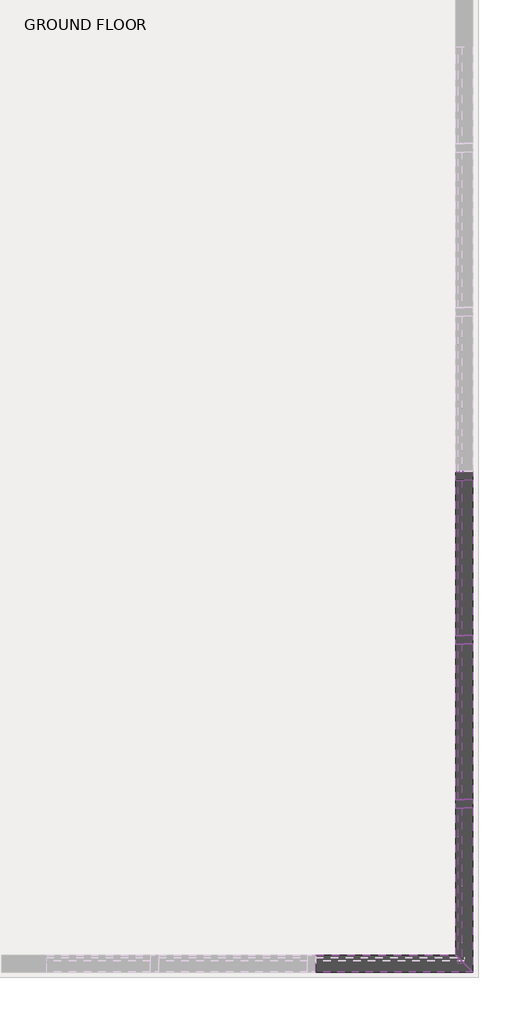
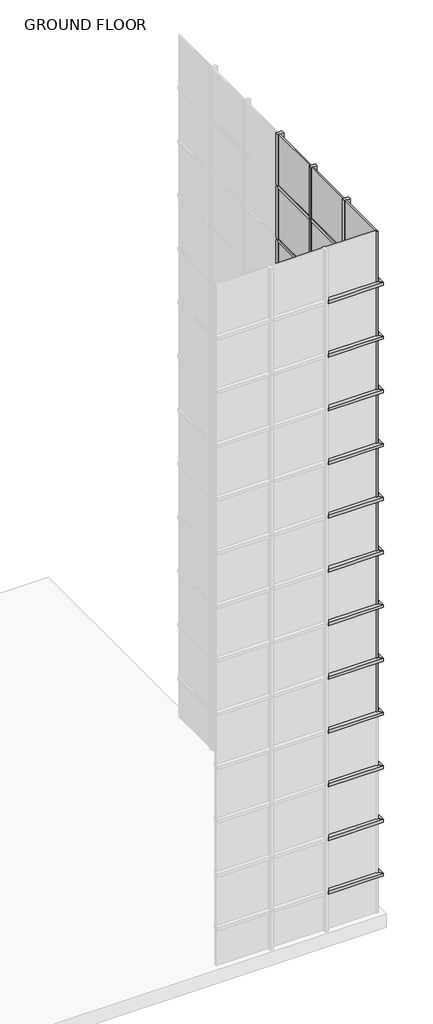
# One storey, part 6 of 16: 87 members, 43 plates.
"""IFC4 building model written with IfcOpenShell, lengths in millimetres."""

from ifc_helpers import new_model, si_unit, origin, place, context, project, spatial, transform, mapped, element, save
from components import member_a361ce75, member_80100a85, member_b860638c, member_31fee25f, member_49b1bc66, system_panel_glazed_49652e9e

model = new_model("IFC4")

# Units and contexts
model_context = context("Model", 3, world=origin())
ifc_project = project(units=[si_unit("LENGTHUNIT", "METRE", prefix="MILLI")], contexts=[model_context])

# Site, building, storey
site = spatial("IfcSite", under=ifc_project)
building = spatial("IfcBuilding", under=site)
storey = spatial("IfcBuildingStorey", under=building, Name="GROUND FLOOR", Elevation=0.0)

# Members
placement = place(None, origin())
member_shape = member_a361ce75(model_context)
element("IfcMember", 1, ObjectType="Rectangular Mullion : 2.5\" x 5\" rectangular", at=placement, inside=storey, context=model_context, shape_type="MappedRepresentation", body=[
    mapped(member_shape, transform((5962.6982466, -5739.2238032, 1168.8884615), x_axis=(0.0, 0.0, 1.0), y_axis=(0.0, -1.0, 0.0), z_axis=(1.0, 0.0, 0.0))),
])
element("IfcMember", 2, ObjectType="Rectangular Mullion : 2.5\" x 5\" rectangular", at=placement, inside=storey, context=model_context, shape_type="MappedRepresentation", body=[
    mapped(member_shape, transform((5962.6982466, -5739.2238032, 2369.5269231), x_axis=(0.0, 0.0, 1.0), y_axis=(0.0, -1.0, 0.0), z_axis=(1.0, 0.0, 0.0))),
])
element("IfcMember", 3, ObjectType="Rectangular Mullion : 2.5\" x 5\" rectangular", at=placement, inside=storey, context=model_context, shape_type="MappedRepresentation", body=[
    mapped(member_shape, transform((5962.6982466, -5739.2238032, 3570.1653846), x_axis=(0.0, 0.0, 1.0), y_axis=(0.0, -1.0, 0.0), z_axis=(1.0, 0.0, 0.0))),
])
element("IfcMember", 4, ObjectType="Rectangular Mullion : 2.5\" x 5\" rectangular", at=placement, inside=storey, context=model_context, shape_type="MappedRepresentation", body=[
    mapped(member_shape, transform((5962.6982466, -5739.2238032, 4770.8038462), x_axis=(0.0, 0.0, 1.0), y_axis=(0.0, -1.0, 0.0), z_axis=(1.0, 0.0, 0.0))),
])
element("IfcMember", 5, ObjectType="Rectangular Mullion : 2.5\" x 5\" rectangular", at=placement, inside=storey, context=model_context, shape_type="MappedRepresentation", body=[
    mapped(member_shape, transform((5962.6982466, -5739.2238032, 5971.4423077), x_axis=(0.0, 0.0, 1.0), y_axis=(0.0, -1.0, 0.0), z_axis=(1.0, 0.0, 0.0))),
])
element("IfcMember", 6, ObjectType="Rectangular Mullion : 2.5\" x 5\" rectangular", at=placement, inside=storey, context=model_context, shape_type="MappedRepresentation", body=[
    mapped(member_shape, transform((5962.6982466, -5739.2238032, 7172.0807692), x_axis=(0.0, 0.0, 1.0), y_axis=(0.0, -1.0, 0.0), z_axis=(1.0, 0.0, 0.0))),
])
element("IfcMember", 7, ObjectType="Rectangular Mullion : 2.5\" x 5\" rectangular", at=placement, inside=storey, context=model_context, shape_type="MappedRepresentation", body=[
    mapped(member_shape, transform((5962.6982466, -5739.2238032, 8372.7192308), x_axis=(0.0, 0.0, 1.0), y_axis=(0.0, -1.0, 0.0), z_axis=(1.0, 0.0, 0.0))),
])
element("IfcMember", 8, ObjectType="Rectangular Mullion : 2.5\" x 5\" rectangular", at=placement, inside=storey, context=model_context, shape_type="MappedRepresentation", body=[
    mapped(member_shape, transform((5962.6982466, -5739.2238032, 9573.3576923), x_axis=(0.0, 0.0, 1.0), y_axis=(0.0, -1.0, 0.0), z_axis=(1.0, 0.0, 0.0))),
])
element("IfcMember", 9, ObjectType="Rectangular Mullion : 2.5\" x 5\" rectangular", at=placement, inside=storey, context=model_context, shape_type="MappedRepresentation", body=[
    mapped(member_shape, transform((5962.6982466, -5739.2238032, 10773.9961538), x_axis=(0.0, 0.0, 1.0), y_axis=(0.0, -1.0, 0.0), z_axis=(1.0, 0.0, 0.0))),
])
element("IfcMember", 10, ObjectType="Rectangular Mullion : 2.5\" x 5\" rectangular", at=placement, inside=storey, context=model_context, shape_type="MappedRepresentation", body=[
    mapped(member_shape, transform((5962.6982466, -5739.2238032, 11974.6346154), x_axis=(0.0, 0.0, 1.0), y_axis=(0.0, -1.0, 0.0), z_axis=(1.0, 0.0, 0.0))),
])
element("IfcMember", 11, ObjectType="Rectangular Mullion : 2.5\" x 5\" rectangular", at=placement, inside=storey, context=model_context, shape_type="MappedRepresentation", body=[
    mapped(member_shape, transform((5962.6982466, -5739.2238032, 13175.2730769), x_axis=(0.0, 0.0, 1.0), y_axis=(0.0, -1.0, 0.0), z_axis=(1.0, 0.0, 0.0))),
])
element("IfcMember", 12, ObjectType="Rectangular Mullion : 2.5\" x 5\" rectangular", at=placement, inside=storey, context=model_context, shape_type="MappedRepresentation", body=[
    mapped(member_shape, transform((5962.6982466, -5739.2238032, 14375.9115385), x_axis=(0.0, 0.0, 1.0), y_axis=(0.0, -1.0, 0.0), z_axis=(1.0, 0.0, 0.0))),
])
member_2_shape = member_80100a85(model_context)
element("IfcMember", 13, ObjectType="Rectangular Mullion : 2.5\" x 5\" rectangular", at=placement, inside=storey, context=model_context, shape_type="MappedRepresentation", body=[
    mapped(member_2_shape, transform((5962.6982466, -4585.428803, 1168.8884615), x_axis=(0.0, 0.0, 1.0), y_axis=(1.0, 0.0, 0.0), z_axis=(0.0, 1.0, 0.0))),
])
element("IfcMember", 14, ObjectType="Rectangular Mullion : 2.5\" x 5\" rectangular", at=placement, inside=storey, context=model_context, shape_type="MappedRepresentation", body=[
    mapped(member_2_shape, transform((5962.6982466, -4585.428803, 2369.5269231), x_axis=(0.0, 0.0, 1.0), y_axis=(1.0, 0.0, 0.0), z_axis=(0.0, 1.0, 0.0))),
])
element("IfcMember", 15, ObjectType="Rectangular Mullion : 2.5\" x 5\" rectangular", at=placement, inside=storey, context=model_context, shape_type="MappedRepresentation", body=[
    mapped(member_2_shape, transform((5962.6982466, -4585.428803, 3570.1653846), x_axis=(0.0, 0.0, 1.0), y_axis=(1.0, 0.0, 0.0), z_axis=(0.0, 1.0, 0.0))),
])
element("IfcMember", 16, ObjectType="Rectangular Mullion : 2.5\" x 5\" rectangular", at=placement, inside=storey, context=model_context, shape_type="MappedRepresentation", body=[
    mapped(member_2_shape, transform((5962.6982466, -4585.428803, 4770.8038462), x_axis=(0.0, 0.0, 1.0), y_axis=(1.0, 0.0, 0.0), z_axis=(0.0, 1.0, 0.0))),
])
element("IfcMember", 17, ObjectType="Rectangular Mullion : 2.5\" x 5\" rectangular", at=placement, inside=storey, context=model_context, shape_type="MappedRepresentation", body=[
    mapped(member_2_shape, transform((5962.6982466, -4585.428803, 5971.4423077), x_axis=(0.0, 0.0, 1.0), y_axis=(1.0, 0.0, 0.0), z_axis=(0.0, 1.0, 0.0))),
])
element("IfcMember", 18, ObjectType="Rectangular Mullion : 2.5\" x 5\" rectangular", at=placement, inside=storey, context=model_context, shape_type="MappedRepresentation", body=[
    mapped(member_2_shape, transform((5962.6982466, -4585.428803, 7172.0807692), x_axis=(0.0, 0.0, 1.0), y_axis=(1.0, 0.0, 0.0), z_axis=(0.0, 1.0, 0.0))),
])
element("IfcMember", 19, ObjectType="Rectangular Mullion : 2.5\" x 5\" rectangular", at=placement, inside=storey, context=model_context, shape_type="MappedRepresentation", body=[
    mapped(member_2_shape, transform((5962.6982466, -4585.428803, 8372.7192308), x_axis=(0.0, 0.0, 1.0), y_axis=(1.0, 0.0, 0.0), z_axis=(0.0, 1.0, 0.0))),
])
element("IfcMember", 20, ObjectType="Rectangular Mullion : 2.5\" x 5\" rectangular", at=placement, inside=storey, context=model_context, shape_type="MappedRepresentation", body=[
    mapped(member_2_shape, transform((5962.6982466, -4585.428803, 9573.3576923), x_axis=(0.0, 0.0, 1.0), y_axis=(1.0, 0.0, 0.0), z_axis=(0.0, 1.0, 0.0))),
])
element("IfcMember", 21, ObjectType="Rectangular Mullion : 2.5\" x 5\" rectangular", at=placement, inside=storey, context=model_context, shape_type="MappedRepresentation", body=[
    mapped(member_2_shape, transform((5962.6982466, -4585.428803, 10773.9961538), x_axis=(0.0, 0.0, 1.0), y_axis=(1.0, 0.0, 0.0), z_axis=(0.0, 1.0, 0.0))),
])
element("IfcMember", 22, ObjectType="Rectangular Mullion : 2.5\" x 5\" rectangular", at=placement, inside=storey, context=model_context, shape_type="MappedRepresentation", body=[
    mapped(member_2_shape, transform((5962.6982466, -4585.428803, 11974.6346154), x_axis=(0.0, 0.0, 1.0), y_axis=(1.0, 0.0, 0.0), z_axis=(0.0, 1.0, 0.0))),
])
element("IfcMember", 23, ObjectType="Rectangular Mullion : 2.5\" x 5\" rectangular", at=placement, inside=storey, context=model_context, shape_type="MappedRepresentation", body=[
    mapped(member_2_shape, transform((5962.6982466, -4585.428803, 13175.2730769), x_axis=(0.0, 0.0, 1.0), y_axis=(1.0, 0.0, 0.0), z_axis=(0.0, 1.0, 0.0))),
])
element("IfcMember", 24, ObjectType="Rectangular Mullion : 2.5\" x 5\" rectangular", at=placement, inside=storey, context=model_context, shape_type="MappedRepresentation", body=[
    mapped(member_2_shape, transform((5962.6982466, -4585.428803, 14375.9115385), x_axis=(0.0, 0.0, 1.0), y_axis=(1.0, 0.0, 0.0), z_axis=(0.0, 1.0, 0.0))),
])
member_3_shape = member_b860638c(model_context)
element("IfcMember", 25, ObjectType="Rectangular Mullion : 2.5\" x 5\" rectangular", at=placement, inside=storey, context=model_context, shape_type="MappedRepresentation", body=[
    mapped(member_3_shape, transform((5962.6982466, -4553.678803, 0.0), x_axis=(0.0, 1.0, 0.0), y_axis=(1.0, 0.0, 0.0), z_axis=(0.0, 0.0, -1.0))),
])
element("IfcMember", 26, ObjectType="Rectangular Mullion : 2.5\" x 5\" rectangular", at=placement, inside=storey, context=model_context, shape_type="MappedRepresentation", body=[
    mapped(member_3_shape, transform((5962.6982466, -3336.383803, 0.0), x_axis=(0.0, 1.0, 0.0), y_axis=(1.0, 0.0, 0.0), z_axis=(0.0, 0.0, -1.0))),
])
element("IfcMember", 27, ObjectType="Rectangular Mullion : 2.5\" x 5\" rectangular", at=placement, inside=storey, context=model_context, shape_type="MappedRepresentation", body=[
    mapped(member_3_shape, transform((5962.6982466, -2119.0888031, 0.0), x_axis=(0.0, 1.0, 0.0), y_axis=(1.0, 0.0, 0.0), z_axis=(0.0, 0.0, -1.0))),
])
member_4_shape = member_31fee25f(model_context)
element("IfcMember", 28, ObjectType="Rectangular Mullion : 2.5\" x 5\" rectangular", at=placement, inside=storey, context=model_context, shape_type="MappedRepresentation", body=[
    mapped(member_4_shape, transform((5962.6982466, -4553.678803, 1168.8884615), x_axis=(0.0, 1.0, 0.0), y_axis=(1.0, 0.0, 0.0), z_axis=(0.0, 0.0, -1.0))),
])
element("IfcMember", 29, ObjectType="Rectangular Mullion : 2.5\" x 5\" rectangular", at=placement, inside=storey, context=model_context, shape_type="MappedRepresentation", body=[
    mapped(member_4_shape, transform((5962.6982466, -3336.383803, 1168.8884615), x_axis=(0.0, 1.0, 0.0), y_axis=(1.0, 0.0, 0.0), z_axis=(0.0, 0.0, -1.0))),
])
element("IfcMember", 30, ObjectType="Rectangular Mullion : 2.5\" x 5\" rectangular", at=placement, inside=storey, context=model_context, shape_type="MappedRepresentation", body=[
    mapped(member_4_shape, transform((5962.6982466, -2119.0888031, 1168.8884615), x_axis=(0.0, 1.0, 0.0), y_axis=(1.0, 0.0, 0.0), z_axis=(0.0, 0.0, -1.0))),
])
element("IfcMember", 31, ObjectType="Rectangular Mullion : 2.5\" x 5\" rectangular", at=placement, inside=storey, context=model_context, shape_type="MappedRepresentation", body=[
    mapped(member_4_shape, transform((5962.6982466, -4553.678803, 2369.5269231), x_axis=(0.0, 1.0, 0.0), y_axis=(1.0, 0.0, 0.0), z_axis=(0.0, 0.0, -1.0))),
])
element("IfcMember", 32, ObjectType="Rectangular Mullion : 2.5\" x 5\" rectangular", at=placement, inside=storey, context=model_context, shape_type="MappedRepresentation", body=[
    mapped(member_4_shape, transform((5962.6982466, -3336.383803, 2369.5269231), x_axis=(0.0, 1.0, 0.0), y_axis=(1.0, 0.0, 0.0), z_axis=(0.0, 0.0, -1.0))),
])
element("IfcMember", 33, ObjectType="Rectangular Mullion : 2.5\" x 5\" rectangular", at=placement, inside=storey, context=model_context, shape_type="MappedRepresentation", body=[
    mapped(member_4_shape, transform((5962.6982466, -2119.0888031, 2369.5269231), x_axis=(0.0, 1.0, 0.0), y_axis=(1.0, 0.0, 0.0), z_axis=(0.0, 0.0, -1.0))),
])
element("IfcMember", 34, ObjectType="Rectangular Mullion : 2.5\" x 5\" rectangular", at=placement, inside=storey, context=model_context, shape_type="MappedRepresentation", body=[
    mapped(member_4_shape, transform((5962.6982466, -4553.678803, 3570.1653846), x_axis=(0.0, 1.0, 0.0), y_axis=(1.0, 0.0, 0.0), z_axis=(0.0, 0.0, -1.0))),
])
element("IfcMember", 35, ObjectType="Rectangular Mullion : 2.5\" x 5\" rectangular", at=placement, inside=storey, context=model_context, shape_type="MappedRepresentation", body=[
    mapped(member_4_shape, transform((5962.6982466, -3336.383803, 3570.1653846), x_axis=(0.0, 1.0, 0.0), y_axis=(1.0, 0.0, 0.0), z_axis=(0.0, 0.0, -1.0))),
])
element("IfcMember", 36, ObjectType="Rectangular Mullion : 2.5\" x 5\" rectangular", at=placement, inside=storey, context=model_context, shape_type="MappedRepresentation", body=[
    mapped(member_4_shape, transform((5962.6982466, -2119.0888031, 3570.1653846), x_axis=(0.0, 1.0, 0.0), y_axis=(1.0, 0.0, 0.0), z_axis=(0.0, 0.0, -1.0))),
])
element("IfcMember", 37, ObjectType="Rectangular Mullion : 2.5\" x 5\" rectangular", at=placement, inside=storey, context=model_context, shape_type="MappedRepresentation", body=[
    mapped(member_4_shape, transform((5962.6982466, -4553.678803, 4770.8038462), x_axis=(0.0, 1.0, 0.0), y_axis=(1.0, 0.0, 0.0), z_axis=(0.0, 0.0, -1.0))),
])
element("IfcMember", 38, ObjectType="Rectangular Mullion : 2.5\" x 5\" rectangular", at=placement, inside=storey, context=model_context, shape_type="MappedRepresentation", body=[
    mapped(member_4_shape, transform((5962.6982466, -3336.383803, 4770.8038462), x_axis=(0.0, 1.0, 0.0), y_axis=(1.0, 0.0, 0.0), z_axis=(0.0, 0.0, -1.0))),
])
element("IfcMember", 39, ObjectType="Rectangular Mullion : 2.5\" x 5\" rectangular", at=placement, inside=storey, context=model_context, shape_type="MappedRepresentation", body=[
    mapped(member_4_shape, transform((5962.6982466, -2119.0888031, 4770.8038462), x_axis=(0.0, 1.0, 0.0), y_axis=(1.0, 0.0, 0.0), z_axis=(0.0, 0.0, -1.0))),
])
element("IfcMember", 40, ObjectType="Rectangular Mullion : 2.5\" x 5\" rectangular", at=placement, inside=storey, context=model_context, shape_type="MappedRepresentation", body=[
    mapped(member_4_shape, transform((5962.6982466, -4553.678803, 5971.4423077), x_axis=(0.0, 1.0, 0.0), y_axis=(1.0, 0.0, 0.0), z_axis=(0.0, 0.0, -1.0))),
])
element("IfcMember", 41, ObjectType="Rectangular Mullion : 2.5\" x 5\" rectangular", at=placement, inside=storey, context=model_context, shape_type="MappedRepresentation", body=[
    mapped(member_4_shape, transform((5962.6982466, -3336.383803, 5971.4423077), x_axis=(0.0, 1.0, 0.0), y_axis=(1.0, 0.0, 0.0), z_axis=(0.0, 0.0, -1.0))),
])
element("IfcMember", 42, ObjectType="Rectangular Mullion : 2.5\" x 5\" rectangular", at=placement, inside=storey, context=model_context, shape_type="MappedRepresentation", body=[
    mapped(member_4_shape, transform((5962.6982466, -2119.0888031, 5971.4423077), x_axis=(0.0, 1.0, 0.0), y_axis=(1.0, 0.0, 0.0), z_axis=(0.0, 0.0, -1.0))),
])
element("IfcMember", 43, ObjectType="Rectangular Mullion : 2.5\" x 5\" rectangular", at=placement, inside=storey, context=model_context, shape_type="MappedRepresentation", body=[
    mapped(member_4_shape, transform((5962.6982466, -4553.678803, 7172.0807692), x_axis=(0.0, 1.0, 0.0), y_axis=(1.0, 0.0, 0.0), z_axis=(0.0, 0.0, -1.0))),
])
element("IfcMember", 44, ObjectType="Rectangular Mullion : 2.5\" x 5\" rectangular", at=placement, inside=storey, context=model_context, shape_type="MappedRepresentation", body=[
    mapped(member_4_shape, transform((5962.6982466, -3336.383803, 7172.0807692), x_axis=(0.0, 1.0, 0.0), y_axis=(1.0, 0.0, 0.0), z_axis=(0.0, 0.0, -1.0))),
])
element("IfcMember", 45, ObjectType="Rectangular Mullion : 2.5\" x 5\" rectangular", at=placement, inside=storey, context=model_context, shape_type="MappedRepresentation", body=[
    mapped(member_4_shape, transform((5962.6982466, -2119.0888031, 7172.0807692), x_axis=(0.0, 1.0, 0.0), y_axis=(1.0, 0.0, 0.0), z_axis=(0.0, 0.0, -1.0))),
])
element("IfcMember", 46, ObjectType="Rectangular Mullion : 2.5\" x 5\" rectangular", at=placement, inside=storey, context=model_context, shape_type="MappedRepresentation", body=[
    mapped(member_4_shape, transform((5962.6982466, -4553.678803, 8372.7192308), x_axis=(0.0, 1.0, 0.0), y_axis=(1.0, 0.0, 0.0), z_axis=(0.0, 0.0, -1.0))),
])
element("IfcMember", 47, ObjectType="Rectangular Mullion : 2.5\" x 5\" rectangular", at=placement, inside=storey, context=model_context, shape_type="MappedRepresentation", body=[
    mapped(member_4_shape, transform((5962.6982466, -3336.383803, 8372.7192308), x_axis=(0.0, 1.0, 0.0), y_axis=(1.0, 0.0, 0.0), z_axis=(0.0, 0.0, -1.0))),
])
element("IfcMember", 48, ObjectType="Rectangular Mullion : 2.5\" x 5\" rectangular", at=placement, inside=storey, context=model_context, shape_type="MappedRepresentation", body=[
    mapped(member_4_shape, transform((5962.6982466, -2119.0888031, 8372.7192308), x_axis=(0.0, 1.0, 0.0), y_axis=(1.0, 0.0, 0.0), z_axis=(0.0, 0.0, -1.0))),
])
element("IfcMember", 49, ObjectType="Rectangular Mullion : 2.5\" x 5\" rectangular", at=placement, inside=storey, context=model_context, shape_type="MappedRepresentation", body=[
    mapped(member_4_shape, transform((5962.6982466, -4553.678803, 9573.3576923), x_axis=(0.0, 1.0, 0.0), y_axis=(1.0, 0.0, 0.0), z_axis=(0.0, 0.0, -1.0))),
])
element("IfcMember", 50, ObjectType="Rectangular Mullion : 2.5\" x 5\" rectangular", at=placement, inside=storey, context=model_context, shape_type="MappedRepresentation", body=[
    mapped(member_4_shape, transform((5962.6982466, -3336.383803, 9573.3576923), x_axis=(0.0, 1.0, 0.0), y_axis=(1.0, 0.0, 0.0), z_axis=(0.0, 0.0, -1.0))),
])
element("IfcMember", 51, ObjectType="Rectangular Mullion : 2.5\" x 5\" rectangular", at=placement, inside=storey, context=model_context, shape_type="MappedRepresentation", body=[
    mapped(member_4_shape, transform((5962.6982466, -2119.0888031, 9573.3576923), x_axis=(0.0, 1.0, 0.0), y_axis=(1.0, 0.0, 0.0), z_axis=(0.0, 0.0, -1.0))),
])
element("IfcMember", 52, ObjectType="Rectangular Mullion : 2.5\" x 5\" rectangular", at=placement, inside=storey, context=model_context, shape_type="MappedRepresentation", body=[
    mapped(member_4_shape, transform((5962.6982466, -4553.678803, 10773.9961538), x_axis=(0.0, 1.0, 0.0), y_axis=(1.0, 0.0, 0.0), z_axis=(0.0, 0.0, -1.0))),
])
element("IfcMember", 53, ObjectType="Rectangular Mullion : 2.5\" x 5\" rectangular", at=placement, inside=storey, context=model_context, shape_type="MappedRepresentation", body=[
    mapped(member_4_shape, transform((5962.6982466, -3336.383803, 10773.9961538), x_axis=(0.0, 1.0, 0.0), y_axis=(1.0, 0.0, 0.0), z_axis=(0.0, 0.0, -1.0))),
])
element("IfcMember", 54, ObjectType="Rectangular Mullion : 2.5\" x 5\" rectangular", at=placement, inside=storey, context=model_context, shape_type="MappedRepresentation", body=[
    mapped(member_4_shape, transform((5962.6982466, -2119.0888031, 10773.9961538), x_axis=(0.0, 1.0, 0.0), y_axis=(1.0, 0.0, 0.0), z_axis=(0.0, 0.0, -1.0))),
])
element("IfcMember", 55, ObjectType="Rectangular Mullion : 2.5\" x 5\" rectangular", at=placement, inside=storey, context=model_context, shape_type="MappedRepresentation", body=[
    mapped(member_4_shape, transform((5962.6982466, -4553.678803, 11974.6346154), x_axis=(0.0, 1.0, 0.0), y_axis=(1.0, 0.0, 0.0), z_axis=(0.0, 0.0, -1.0))),
])
element("IfcMember", 56, ObjectType="Rectangular Mullion : 2.5\" x 5\" rectangular", at=placement, inside=storey, context=model_context, shape_type="MappedRepresentation", body=[
    mapped(member_4_shape, transform((5962.6982466, -3336.383803, 11974.6346154), x_axis=(0.0, 1.0, 0.0), y_axis=(1.0, 0.0, 0.0), z_axis=(0.0, 0.0, -1.0))),
])
element("IfcMember", 57, ObjectType="Rectangular Mullion : 2.5\" x 5\" rectangular", at=placement, inside=storey, context=model_context, shape_type="MappedRepresentation", body=[
    mapped(member_4_shape, transform((5962.6982466, -2119.0888031, 11974.6346154), x_axis=(0.0, 1.0, 0.0), y_axis=(1.0, 0.0, 0.0), z_axis=(0.0, 0.0, -1.0))),
])
element("IfcMember", 58, ObjectType="Rectangular Mullion : 2.5\" x 5\" rectangular", at=placement, inside=storey, context=model_context, shape_type="MappedRepresentation", body=[
    mapped(member_4_shape, transform((5962.6982466, -4553.678803, 13175.2730769), x_axis=(0.0, 1.0, 0.0), y_axis=(1.0, 0.0, 0.0), z_axis=(0.0, 0.0, -1.0))),
])
element("IfcMember", 59, ObjectType="Rectangular Mullion : 2.5\" x 5\" rectangular", at=placement, inside=storey, context=model_context, shape_type="MappedRepresentation", body=[
    mapped(member_4_shape, transform((5962.6982466, -3336.383803, 13175.2730769), x_axis=(0.0, 1.0, 0.0), y_axis=(1.0, 0.0, 0.0), z_axis=(0.0, 0.0, -1.0))),
])
element("IfcMember", 60, ObjectType="Rectangular Mullion : 2.5\" x 5\" rectangular", at=placement, inside=storey, context=model_context, shape_type="MappedRepresentation", body=[
    mapped(member_4_shape, transform((5962.6982466, -2119.0888031, 13175.2730769), x_axis=(0.0, 1.0, 0.0), y_axis=(1.0, 0.0, 0.0), z_axis=(0.0, 0.0, -1.0))),
])
element("IfcMember", 61, ObjectType="Rectangular Mullion : 2.5\" x 5\" rectangular", at=placement, inside=storey, context=model_context, shape_type="MappedRepresentation", body=[
    mapped(member_3_shape, transform((5962.6982466, -4553.678803, 14375.9115385), x_axis=(0.0, 1.0, 0.0), y_axis=(1.0, 0.0, 0.0), z_axis=(0.0, 0.0, -1.0))),
])
element("IfcMember", 62, ObjectType="Rectangular Mullion : 2.5\" x 5\" rectangular", at=placement, inside=storey, context=model_context, shape_type="MappedRepresentation", body=[
    mapped(member_3_shape, transform((5962.6982466, -3336.383803, 14375.9115385), x_axis=(0.0, 1.0, 0.0), y_axis=(1.0, 0.0, 0.0), z_axis=(0.0, 0.0, -1.0))),
])
element("IfcMember", 63, ObjectType="Rectangular Mullion : 2.5\" x 5\" rectangular", at=placement, inside=storey, context=model_context, shape_type="MappedRepresentation", body=[
    mapped(member_3_shape, transform((5962.6982466, -2119.0888031, 14375.9115385), x_axis=(0.0, 1.0, 0.0), y_axis=(1.0, 0.0, 0.0), z_axis=(0.0, 0.0, -1.0))),
])
member_5_shape = member_49b1bc66(model_context)
element("IfcMember", 64, ObjectType="Rectangular Mullion : 2.5\" x 5\" rectangular", at=placement, inside=storey, context=model_context, shape_type="MappedRepresentation", body=[
    mapped(member_5_shape, transform((5962.6982466, -3368.133803, 1168.8884615), x_axis=(0.0, 0.0, 1.0), y_axis=(1.0, 0.0, 0.0), z_axis=(0.0, 1.0, 0.0))),
])
element("IfcMember", 65, ObjectType="Rectangular Mullion : 2.5\" x 5\" rectangular", at=placement, inside=storey, context=model_context, shape_type="MappedRepresentation", body=[
    mapped(member_5_shape, transform((5962.6982466, -2150.8388031, 1168.8884615), x_axis=(0.0, 0.0, 1.0), y_axis=(1.0, 0.0, 0.0), z_axis=(0.0, 1.0, 0.0))),
])
element("IfcMember", 66, ObjectType="Rectangular Mullion : 2.5\" x 5\" rectangular", at=placement, inside=storey, context=model_context, shape_type="MappedRepresentation", body=[
    mapped(member_5_shape, transform((5962.6982466, -3368.133803, 2369.5269231), x_axis=(0.0, 0.0, 1.0), y_axis=(1.0, 0.0, 0.0), z_axis=(0.0, 1.0, 0.0))),
])
element("IfcMember", 67, ObjectType="Rectangular Mullion : 2.5\" x 5\" rectangular", at=placement, inside=storey, context=model_context, shape_type="MappedRepresentation", body=[
    mapped(member_5_shape, transform((5962.6982466, -2150.8388031, 2369.5269231), x_axis=(0.0, 0.0, 1.0), y_axis=(1.0, 0.0, 0.0), z_axis=(0.0, 1.0, 0.0))),
])
element("IfcMember", 68, ObjectType="Rectangular Mullion : 2.5\" x 5\" rectangular", at=placement, inside=storey, context=model_context, shape_type="MappedRepresentation", body=[
    mapped(member_5_shape, transform((5962.6982466, -3368.133803, 3570.1653846), x_axis=(0.0, 0.0, 1.0), y_axis=(1.0, 0.0, 0.0), z_axis=(0.0, 1.0, 0.0))),
])
element("IfcMember", 69, ObjectType="Rectangular Mullion : 2.5\" x 5\" rectangular", at=placement, inside=storey, context=model_context, shape_type="MappedRepresentation", body=[
    mapped(member_5_shape, transform((5962.6982466, -2150.8388031, 3570.1653846), x_axis=(0.0, 0.0, 1.0), y_axis=(1.0, 0.0, 0.0), z_axis=(0.0, 1.0, 0.0))),
])
element("IfcMember", 70, ObjectType="Rectangular Mullion : 2.5\" x 5\" rectangular", at=placement, inside=storey, context=model_context, shape_type="MappedRepresentation", body=[
    mapped(member_5_shape, transform((5962.6982466, -3368.133803, 4770.8038462), x_axis=(0.0, 0.0, 1.0), y_axis=(1.0, 0.0, 0.0), z_axis=(0.0, 1.0, 0.0))),
])
element("IfcMember", 71, ObjectType="Rectangular Mullion : 2.5\" x 5\" rectangular", at=placement, inside=storey, context=model_context, shape_type="MappedRepresentation", body=[
    mapped(member_5_shape, transform((5962.6982466, -2150.8388031, 4770.8038462), x_axis=(0.0, 0.0, 1.0), y_axis=(1.0, 0.0, 0.0), z_axis=(0.0, 1.0, 0.0))),
])
element("IfcMember", 72, ObjectType="Rectangular Mullion : 2.5\" x 5\" rectangular", at=placement, inside=storey, context=model_context, shape_type="MappedRepresentation", body=[
    mapped(member_5_shape, transform((5962.6982466, -3368.133803, 5971.4423077), x_axis=(0.0, 0.0, 1.0), y_axis=(1.0, 0.0, 0.0), z_axis=(0.0, 1.0, 0.0))),
])
element("IfcMember", 73, ObjectType="Rectangular Mullion : 2.5\" x 5\" rectangular", at=placement, inside=storey, context=model_context, shape_type="MappedRepresentation", body=[
    mapped(member_5_shape, transform((5962.6982466, -2150.8388031, 5971.4423077), x_axis=(0.0, 0.0, 1.0), y_axis=(1.0, 0.0, 0.0), z_axis=(0.0, 1.0, 0.0))),
])
element("IfcMember", 74, ObjectType="Rectangular Mullion : 2.5\" x 5\" rectangular", at=placement, inside=storey, context=model_context, shape_type="MappedRepresentation", body=[
    mapped(member_5_shape, transform((5962.6982466, -3368.133803, 7172.0807692), x_axis=(0.0, 0.0, 1.0), y_axis=(1.0, 0.0, 0.0), z_axis=(0.0, 1.0, 0.0))),
])
element("IfcMember", 75, ObjectType="Rectangular Mullion : 2.5\" x 5\" rectangular", at=placement, inside=storey, context=model_context, shape_type="MappedRepresentation", body=[
    mapped(member_5_shape, transform((5962.6982466, -2150.8388031, 7172.0807692), x_axis=(0.0, 0.0, 1.0), y_axis=(1.0, 0.0, 0.0), z_axis=(0.0, 1.0, 0.0))),
])
element("IfcMember", 76, ObjectType="Rectangular Mullion : 2.5\" x 5\" rectangular", at=placement, inside=storey, context=model_context, shape_type="MappedRepresentation", body=[
    mapped(member_5_shape, transform((5962.6982466, -3368.133803, 8372.7192308), x_axis=(0.0, 0.0, 1.0), y_axis=(1.0, 0.0, 0.0), z_axis=(0.0, 1.0, 0.0))),
])
element("IfcMember", 77, ObjectType="Rectangular Mullion : 2.5\" x 5\" rectangular", at=placement, inside=storey, context=model_context, shape_type="MappedRepresentation", body=[
    mapped(member_5_shape, transform((5962.6982466, -2150.8388031, 8372.7192308), x_axis=(0.0, 0.0, 1.0), y_axis=(1.0, 0.0, 0.0), z_axis=(0.0, 1.0, 0.0))),
])
element("IfcMember", 78, ObjectType="Rectangular Mullion : 2.5\" x 5\" rectangular", at=placement, inside=storey, context=model_context, shape_type="MappedRepresentation", body=[
    mapped(member_5_shape, transform((5962.6982466, -3368.133803, 9573.3576923), x_axis=(0.0, 0.0, 1.0), y_axis=(1.0, 0.0, 0.0), z_axis=(0.0, 1.0, 0.0))),
])
element("IfcMember", 79, ObjectType="Rectangular Mullion : 2.5\" x 5\" rectangular", at=placement, inside=storey, context=model_context, shape_type="MappedRepresentation", body=[
    mapped(member_5_shape, transform((5962.6982466, -2150.8388031, 9573.3576923), x_axis=(0.0, 0.0, 1.0), y_axis=(1.0, 0.0, 0.0), z_axis=(0.0, 1.0, 0.0))),
])
element("IfcMember", 80, ObjectType="Rectangular Mullion : 2.5\" x 5\" rectangular", at=placement, inside=storey, context=model_context, shape_type="MappedRepresentation", body=[
    mapped(member_5_shape, transform((5962.6982466, -3368.133803, 10773.9961538), x_axis=(0.0, 0.0, 1.0), y_axis=(1.0, 0.0, 0.0), z_axis=(0.0, 1.0, 0.0))),
])
element("IfcMember", 81, ObjectType="Rectangular Mullion : 2.5\" x 5\" rectangular", at=placement, inside=storey, context=model_context, shape_type="MappedRepresentation", body=[
    mapped(member_5_shape, transform((5962.6982466, -2150.8388031, 10773.9961538), x_axis=(0.0, 0.0, 1.0), y_axis=(1.0, 0.0, 0.0), z_axis=(0.0, 1.0, 0.0))),
])
element("IfcMember", 82, ObjectType="Rectangular Mullion : 2.5\" x 5\" rectangular", at=placement, inside=storey, context=model_context, shape_type="MappedRepresentation", body=[
    mapped(member_5_shape, transform((5962.6982466, -3368.133803, 11974.6346154), x_axis=(0.0, 0.0, 1.0), y_axis=(1.0, 0.0, 0.0), z_axis=(0.0, 1.0, 0.0))),
])
element("IfcMember", 83, ObjectType="Rectangular Mullion : 2.5\" x 5\" rectangular", at=placement, inside=storey, context=model_context, shape_type="MappedRepresentation", body=[
    mapped(member_5_shape, transform((5962.6982466, -2150.8388031, 11974.6346154), x_axis=(0.0, 0.0, 1.0), y_axis=(1.0, 0.0, 0.0), z_axis=(0.0, 1.0, 0.0))),
])
element("IfcMember", 84, ObjectType="Rectangular Mullion : 2.5\" x 5\" rectangular", at=placement, inside=storey, context=model_context, shape_type="MappedRepresentation", body=[
    mapped(member_5_shape, transform((5962.6982466, -3368.133803, 13175.2730769), x_axis=(0.0, 0.0, 1.0), y_axis=(1.0, 0.0, 0.0), z_axis=(0.0, 1.0, 0.0))),
])
element("IfcMember", 85, ObjectType="Rectangular Mullion : 2.5\" x 5\" rectangular", at=placement, inside=storey, context=model_context, shape_type="MappedRepresentation", body=[
    mapped(member_5_shape, transform((5962.6982466, -2150.8388031, 13175.2730769), x_axis=(0.0, 0.0, 1.0), y_axis=(1.0, 0.0, 0.0), z_axis=(0.0, 1.0, 0.0))),
])
element("IfcMember", 86, ObjectType="Rectangular Mullion : 2.5\" x 5\" rectangular", at=placement, inside=storey, context=model_context, shape_type="MappedRepresentation", body=[
    mapped(member_5_shape, transform((5962.6982466, -3368.133803, 14375.9115385), x_axis=(0.0, 0.0, 1.0), y_axis=(1.0, 0.0, 0.0), z_axis=(0.0, 1.0, 0.0))),
])
element("IfcMember", 87, ObjectType="Rectangular Mullion : 2.5\" x 5\" rectangular", at=placement, inside=storey, context=model_context, shape_type="MappedRepresentation", body=[
    mapped(member_5_shape, transform((5962.6982466, -2150.8388031, 14375.9115385), x_axis=(0.0, 0.0, 1.0), y_axis=(1.0, 0.0, 0.0), z_axis=(0.0, 1.0, 0.0))),
])

# Plates
system_panel_glazed_shape = system_panel_glazed_49652e9e(model_context)
element("IfcPlate", 88, ObjectType="System Panel : Glazed", at=placement, inside=storey, context=model_context, shape_type="MappedRepresentation", body=[
    mapped(system_panel_glazed_shape, transform((5962.6982466, -3945.031303, 0.0), x_axis=(0.0, 1.0, 0.0), y_axis=(-1.0, 0.0, 0.0), z_axis=(0.0, 0.0, 1.0))),
])
element("IfcPlate", 89, ObjectType="System Panel : Glazed", at=placement, inside=storey, context=model_context, shape_type="MappedRepresentation", body=[
    mapped(system_panel_glazed_shape, transform((5962.6982466, -2727.7363031, 0.0), x_axis=(0.0, 1.0, 0.0), y_axis=(-1.0, 0.0, 0.0), z_axis=(0.0, 0.0, 1.0))),
])
element("IfcPlate", 90, ObjectType="System Panel : Glazed", at=placement, inside=storey, context=model_context, shape_type="MappedRepresentation", body=[
    mapped(system_panel_glazed_shape, transform((5962.6982466, -1510.4413031, 0.0), x_axis=(0.0, 1.0, 0.0), y_axis=(-1.0, 0.0, 0.0), z_axis=(0.0, 0.0, 1.0))),
])
element("IfcPlate", 91, ObjectType="System Panel : Glazed", at=placement, inside=storey, context=model_context, shape_type="MappedRepresentation", body=[
    mapped(system_panel_glazed_shape, transform((5962.6982466, -3945.031303, 1200.6384615), x_axis=(0.0, 1.0, 0.0), y_axis=(-1.0, 0.0, 0.0), z_axis=(0.0, 0.0, 1.0))),
])
element("IfcPlate", 92, ObjectType="System Panel : Glazed", at=placement, inside=storey, context=model_context, shape_type="MappedRepresentation", body=[
    mapped(system_panel_glazed_shape, transform((5962.6982466, -2727.7363031, 1200.6384615), x_axis=(0.0, 1.0, 0.0), y_axis=(-1.0, 0.0, 0.0), z_axis=(0.0, 0.0, 1.0))),
])
element("IfcPlate", 93, ObjectType="System Panel : Glazed", at=placement, inside=storey, context=model_context, shape_type="MappedRepresentation", body=[
    mapped(system_panel_glazed_shape, transform((5962.6982466, -1510.4413031, 1200.6384615), x_axis=(0.0, 1.0, 0.0), y_axis=(-1.0, 0.0, 0.0), z_axis=(0.0, 0.0, 1.0))),
])
element("IfcPlate", 94, ObjectType="System Panel : Glazed", at=placement, inside=storey, context=model_context, shape_type="MappedRepresentation", body=[
    mapped(system_panel_glazed_shape, transform((5962.6982466, -3945.031303, 2401.2769231), x_axis=(0.0, 1.0, 0.0), y_axis=(-1.0, 0.0, 0.0), z_axis=(0.0, 0.0, 1.0))),
])
element("IfcPlate", 95, ObjectType="System Panel : Glazed", at=placement, inside=storey, context=model_context, shape_type="MappedRepresentation", body=[
    mapped(system_panel_glazed_shape, transform((5962.6982466, -2727.7363031, 2401.2769231), x_axis=(0.0, 1.0, 0.0), y_axis=(-1.0, 0.0, 0.0), z_axis=(0.0, 0.0, 1.0))),
])
element("IfcPlate", 96, ObjectType="System Panel : Glazed", at=placement, inside=storey, context=model_context, shape_type="MappedRepresentation", body=[
    mapped(system_panel_glazed_shape, transform((5962.6982466, -1510.4413031, 2401.2769231), x_axis=(0.0, 1.0, 0.0), y_axis=(-1.0, 0.0, 0.0), z_axis=(0.0, 0.0, 1.0))),
])
element("IfcPlate", 97, ObjectType="System Panel : Glazed", at=placement, inside=storey, context=model_context, shape_type="MappedRepresentation", body=[
    mapped(system_panel_glazed_shape, transform((5962.6982466, -3945.031303, 3601.9153846), x_axis=(0.0, 1.0, 0.0), y_axis=(-1.0, 0.0, 0.0), z_axis=(0.0, 0.0, 1.0))),
])
element("IfcPlate", 98, ObjectType="System Panel : Glazed", at=placement, inside=storey, context=model_context, shape_type="MappedRepresentation", body=[
    mapped(system_panel_glazed_shape, transform((5962.6982466, -2727.7363031, 3601.9153846), x_axis=(0.0, 1.0, 0.0), y_axis=(-1.0, 0.0, 0.0), z_axis=(0.0, 0.0, 1.0))),
])
element("IfcPlate", 99, ObjectType="System Panel : Glazed", at=placement, inside=storey, context=model_context, shape_type="MappedRepresentation", body=[
    mapped(system_panel_glazed_shape, transform((5962.6982466, -1510.4413031, 3601.9153846), x_axis=(0.0, 1.0, 0.0), y_axis=(-1.0, 0.0, 0.0), z_axis=(0.0, 0.0, 1.0))),
])
element("IfcPlate", 100, ObjectType="System Panel : Glazed", at=placement, inside=storey, context=model_context, shape_type="MappedRepresentation", body=[
    mapped(system_panel_glazed_shape, transform((5962.6982466, -5162.3263031, 4802.5538462), x_axis=(0.0, 1.0, 0.0), y_axis=(-1.0, 0.0, 0.0), z_axis=(0.0, 0.0, 1.0))),
])
element("IfcPlate", 101, ObjectType="System Panel : Glazed", at=placement, inside=storey, context=model_context, shape_type="MappedRepresentation", body=[
    mapped(system_panel_glazed_shape, transform((5962.6982466, -3945.031303, 4802.5538462), x_axis=(0.0, 1.0, 0.0), y_axis=(-1.0, 0.0, 0.0), z_axis=(0.0, 0.0, 1.0))),
])
element("IfcPlate", 102, ObjectType="System Panel : Glazed", at=placement, inside=storey, context=model_context, shape_type="MappedRepresentation", body=[
    mapped(system_panel_glazed_shape, transform((5962.6982466, -2727.7363031, 4802.5538462), x_axis=(0.0, 1.0, 0.0), y_axis=(-1.0, 0.0, 0.0), z_axis=(0.0, 0.0, 1.0))),
])
element("IfcPlate", 103, ObjectType="System Panel : Glazed", at=placement, inside=storey, context=model_context, shape_type="MappedRepresentation", body=[
    mapped(system_panel_glazed_shape, transform((5962.6982466, -1510.4413031, 4802.5538462), x_axis=(0.0, 1.0, 0.0), y_axis=(-1.0, 0.0, 0.0), z_axis=(0.0, 0.0, 1.0))),
])
element("IfcPlate", 104, ObjectType="System Panel : Glazed", at=placement, inside=storey, context=model_context, shape_type="MappedRepresentation", body=[
    mapped(system_panel_glazed_shape, transform((5962.6982466, -5162.3263031, 6003.1923077), x_axis=(0.0, 1.0, 0.0), y_axis=(-1.0, 0.0, 0.0), z_axis=(0.0, 0.0, 1.0))),
])
element("IfcPlate", 105, ObjectType="System Panel : Glazed", at=placement, inside=storey, context=model_context, shape_type="MappedRepresentation", body=[
    mapped(system_panel_glazed_shape, transform((5962.6982466, -3945.031303, 6003.1923077), x_axis=(0.0, 1.0, 0.0), y_axis=(-1.0, 0.0, 0.0), z_axis=(0.0, 0.0, 1.0))),
])
element("IfcPlate", 106, ObjectType="System Panel : Glazed", at=placement, inside=storey, context=model_context, shape_type="MappedRepresentation", body=[
    mapped(system_panel_glazed_shape, transform((5962.6982466, -2727.7363031, 6003.1923077), x_axis=(0.0, 1.0, 0.0), y_axis=(-1.0, 0.0, 0.0), z_axis=(0.0, 0.0, 1.0))),
])
element("IfcPlate", 107, ObjectType="System Panel : Glazed", at=placement, inside=storey, context=model_context, shape_type="MappedRepresentation", body=[
    mapped(system_panel_glazed_shape, transform((5962.6982466, -1510.4413031, 6003.1923077), x_axis=(0.0, 1.0, 0.0), y_axis=(-1.0, 0.0, 0.0), z_axis=(0.0, 0.0, 1.0))),
])
element("IfcPlate", 108, ObjectType="System Panel : Glazed", at=placement, inside=storey, context=model_context, shape_type="MappedRepresentation", body=[
    mapped(system_panel_glazed_shape, transform((5962.6982466, -5162.3263031, 7203.8307692), x_axis=(0.0, 1.0, 0.0), y_axis=(-1.0, 0.0, 0.0), z_axis=(0.0, 0.0, 1.0))),
])
element("IfcPlate", 109, ObjectType="System Panel : Glazed", at=placement, inside=storey, context=model_context, shape_type="MappedRepresentation", body=[
    mapped(system_panel_glazed_shape, transform((5962.6982466, -3945.031303, 7203.8307692), x_axis=(0.0, 1.0, 0.0), y_axis=(-1.0, 0.0, 0.0), z_axis=(0.0, 0.0, 1.0))),
])
element("IfcPlate", 110, ObjectType="System Panel : Glazed", at=placement, inside=storey, context=model_context, shape_type="MappedRepresentation", body=[
    mapped(system_panel_glazed_shape, transform((5962.6982466, -2727.7363031, 7203.8307692), x_axis=(0.0, 1.0, 0.0), y_axis=(-1.0, 0.0, 0.0), z_axis=(0.0, 0.0, 1.0))),
])
element("IfcPlate", 111, ObjectType="System Panel : Glazed", at=placement, inside=storey, context=model_context, shape_type="MappedRepresentation", body=[
    mapped(system_panel_glazed_shape, transform((5962.6982466, -1510.4413031, 7203.8307692), x_axis=(0.0, 1.0, 0.0), y_axis=(-1.0, 0.0, 0.0), z_axis=(0.0, 0.0, 1.0))),
])
element("IfcPlate", 112, ObjectType="System Panel : Glazed", at=placement, inside=storey, context=model_context, shape_type="MappedRepresentation", body=[
    mapped(system_panel_glazed_shape, transform((5962.6982466, -5162.3263031, 8404.4692308), x_axis=(0.0, 1.0, 0.0), y_axis=(-1.0, 0.0, 0.0), z_axis=(0.0, 0.0, 1.0))),
])
element("IfcPlate", 113, ObjectType="System Panel : Glazed", at=placement, inside=storey, context=model_context, shape_type="MappedRepresentation", body=[
    mapped(system_panel_glazed_shape, transform((5962.6982466, -3945.031303, 8404.4692308), x_axis=(0.0, 1.0, 0.0), y_axis=(-1.0, 0.0, 0.0), z_axis=(0.0, 0.0, 1.0))),
])
element("IfcPlate", 114, ObjectType="System Panel : Glazed", at=placement, inside=storey, context=model_context, shape_type="MappedRepresentation", body=[
    mapped(system_panel_glazed_shape, transform((5962.6982466, -2727.7363031, 8404.4692308), x_axis=(0.0, 1.0, 0.0), y_axis=(-1.0, 0.0, 0.0), z_axis=(0.0, 0.0, 1.0))),
])
element("IfcPlate", 115, ObjectType="System Panel : Glazed", at=placement, inside=storey, context=model_context, shape_type="MappedRepresentation", body=[
    mapped(system_panel_glazed_shape, transform((5962.6982466, -1510.4413031, 8404.4692308), x_axis=(0.0, 1.0, 0.0), y_axis=(-1.0, 0.0, 0.0), z_axis=(0.0, 0.0, 1.0))),
])
element("IfcPlate", 116, ObjectType="System Panel : Glazed", at=placement, inside=storey, context=model_context, shape_type="MappedRepresentation", body=[
    mapped(system_panel_glazed_shape, transform((5962.6982466, -5162.3263031, 9605.1076923), x_axis=(0.0, 1.0, 0.0), y_axis=(-1.0, 0.0, 0.0), z_axis=(0.0, 0.0, 1.0))),
])
element("IfcPlate", 117, ObjectType="System Panel : Glazed", at=placement, inside=storey, context=model_context, shape_type="MappedRepresentation", body=[
    mapped(system_panel_glazed_shape, transform((5962.6982466, -3945.031303, 9605.1076923), x_axis=(0.0, 1.0, 0.0), y_axis=(-1.0, 0.0, 0.0), z_axis=(0.0, 0.0, 1.0))),
])
element("IfcPlate", 118, ObjectType="System Panel : Glazed", at=placement, inside=storey, context=model_context, shape_type="MappedRepresentation", body=[
    mapped(system_panel_glazed_shape, transform((5962.6982466, -2727.7363031, 9605.1076923), x_axis=(0.0, 1.0, 0.0), y_axis=(-1.0, 0.0, 0.0), z_axis=(0.0, 0.0, 1.0))),
])
element("IfcPlate", 119, ObjectType="System Panel : Glazed", at=placement, inside=storey, context=model_context, shape_type="MappedRepresentation", body=[
    mapped(system_panel_glazed_shape, transform((5962.6982466, -5162.3263031, 10805.7461538), x_axis=(0.0, 1.0, 0.0), y_axis=(-1.0, 0.0, 0.0), z_axis=(0.0, 0.0, 1.0))),
])
element("IfcPlate", 120, ObjectType="System Panel : Glazed", at=placement, inside=storey, context=model_context, shape_type="MappedRepresentation", body=[
    mapped(system_panel_glazed_shape, transform((5962.6982466, -3945.031303, 10805.7461538), x_axis=(0.0, 1.0, 0.0), y_axis=(-1.0, 0.0, 0.0), z_axis=(0.0, 0.0, 1.0))),
])
element("IfcPlate", 121, ObjectType="System Panel : Glazed", at=placement, inside=storey, context=model_context, shape_type="MappedRepresentation", body=[
    mapped(system_panel_glazed_shape, transform((5962.6982466, -2727.7363031, 10805.7461538), x_axis=(0.0, 1.0, 0.0), y_axis=(-1.0, 0.0, 0.0), z_axis=(0.0, 0.0, 1.0))),
])
element("IfcPlate", 122, ObjectType="System Panel : Glazed", at=placement, inside=storey, context=model_context, shape_type="MappedRepresentation", body=[
    mapped(system_panel_glazed_shape, transform((5962.6982466, -5162.3263031, 12006.3846154), x_axis=(0.0, 1.0, 0.0), y_axis=(-1.0, 0.0, 0.0), z_axis=(0.0, 0.0, 1.0))),
])
element("IfcPlate", 123, ObjectType="System Panel : Glazed", at=placement, inside=storey, context=model_context, shape_type="MappedRepresentation", body=[
    mapped(system_panel_glazed_shape, transform((5962.6982466, -3945.031303, 12006.3846154), x_axis=(0.0, 1.0, 0.0), y_axis=(-1.0, 0.0, 0.0), z_axis=(0.0, 0.0, 1.0))),
])
element("IfcPlate", 124, ObjectType="System Panel : Glazed", at=placement, inside=storey, context=model_context, shape_type="MappedRepresentation", body=[
    mapped(system_panel_glazed_shape, transform((5962.6982466, -2727.7363031, 12006.3846154), x_axis=(0.0, 1.0, 0.0), y_axis=(-1.0, 0.0, 0.0), z_axis=(0.0, 0.0, 1.0))),
])
element("IfcPlate", 125, ObjectType="System Panel : Glazed", at=placement, inside=storey, context=model_context, shape_type="MappedRepresentation", body=[
    mapped(system_panel_glazed_shape, transform((5962.6982466, -5162.3263031, 13207.0230769), x_axis=(0.0, 1.0, 0.0), y_axis=(-1.0, 0.0, 0.0), z_axis=(0.0, 0.0, 1.0))),
])
element("IfcPlate", 126, ObjectType="System Panel : Glazed", at=placement, inside=storey, context=model_context, shape_type="MappedRepresentation", body=[
    mapped(system_panel_glazed_shape, transform((5962.6982466, -3945.031303, 13207.0230769), x_axis=(0.0, 1.0, 0.0), y_axis=(-1.0, 0.0, 0.0), z_axis=(0.0, 0.0, 1.0))),
])
element("IfcPlate", 127, ObjectType="System Panel : Glazed", at=placement, inside=storey, context=model_context, shape_type="MappedRepresentation", body=[
    mapped(system_panel_glazed_shape, transform((5962.6982466, -2727.7363031, 13207.0230769), x_axis=(0.0, 1.0, 0.0), y_axis=(-1.0, 0.0, 0.0), z_axis=(0.0, 0.0, 1.0))),
])
element("IfcPlate", 128, ObjectType="System Panel : Glazed", at=placement, inside=storey, context=model_context, shape_type="MappedRepresentation", body=[
    mapped(system_panel_glazed_shape, transform((5962.6982466, -5162.3263031, 14407.6615385), x_axis=(0.0, 1.0, 0.0), y_axis=(-1.0, 0.0, 0.0), z_axis=(0.0, 0.0, 1.0))),
])
element("IfcPlate", 129, ObjectType="System Panel : Glazed", at=placement, inside=storey, context=model_context, shape_type="MappedRepresentation", body=[
    mapped(system_panel_glazed_shape, transform((5962.6982466, -3945.031303, 14407.6615385), x_axis=(0.0, 1.0, 0.0), y_axis=(-1.0, 0.0, 0.0), z_axis=(0.0, 0.0, 1.0))),
])
element("IfcPlate", 130, ObjectType="System Panel : Glazed", at=placement, inside=storey, context=model_context, shape_type="MappedRepresentation", body=[
    mapped(system_panel_glazed_shape, transform((5962.6982466, -2727.7363031, 14407.6615385), x_axis=(0.0, 1.0, 0.0), y_axis=(-1.0, 0.0, 0.0), z_axis=(0.0, 0.0, 1.0))),
])

save(model, "model.ifc")

# Revit data of these elements
# Type "Rectangular Mullion : 2.5\" x 5\" rectangular"
#   built-in parameter 1007304 = 0.416667 (stored number, unit not read)
#   built-in parameter 1007301 = 0.104167 (stored number, unit not read)
#   built-in parameter 1007300 = 0.104167 (stored number, unit not read)
# Type "System Panel : Glazed"
#   Construction Type Id = "GSP4R"
#   Analytic Construction = "1/8 in Pilkington single glazing"
#   Visual Light Transmittance = 0.9
#   Solar Heat Gain Coefficient = 0.86
#   Heat Transfer Coefficient (U) = 1.18115 BTU/(h·ft²·°F)
#   Define Thermal Properties by = 1
# Elements 1, 2, 3, 4, 5, 6, 7, 8, 9, 10, 11, 12, 13, 14, 15, 16, 17, 18, 19, 20, 21, 22, 23, 24, 25, 26, 27, 28, 29, 30, 31, 32, 33, 34, 35, 36, 37, 38, 39, 40, 41, 42, 43, 44, 45, 46, 47, 48, 49, 50, 51, 52, 53, 54, 55, 56, 57, 58, 59, 60, 61, 62, 63, 64, 65, 66, 67, 68, 69, 70, 71, 72, 73, 74, 75, 76, 77, 78, 79, 80, 81, 82, 83, 84, 85, 86, 87 (IfcMember, "Rectangular Mullion : 2.5\" x 5\" rectangular")
#   Phase Created = New Construction
#   Materials on its faces: "Aluminum"
# Elements 88, 89, 90, 91, 92, 93, 94, 95, 96, 97, 98, 99, 100, 101, 102, 103, 104, 105, 106, 107, 108, 109, 110, 111, 112, 113, 114, 115, 116, 117, 118, 119, 120, 121, 122, 123, 124, 125, 126, 127, 128, 129, 130 (IfcPlate, "System Panel : Glazed")
#   Phase Created = New Construction
#   Materials on its faces: "Glass"
# Materials
#   "Aluminum": class "Metal", colour RGB 247 247 247, transparency 0, Description = "Aluminum 6061", Cost = 0
#   "Glass": class "Glass", colour RGB 0 128 192, transparency 0.75, Description = "Soda Lime Glass", Cost = 0
